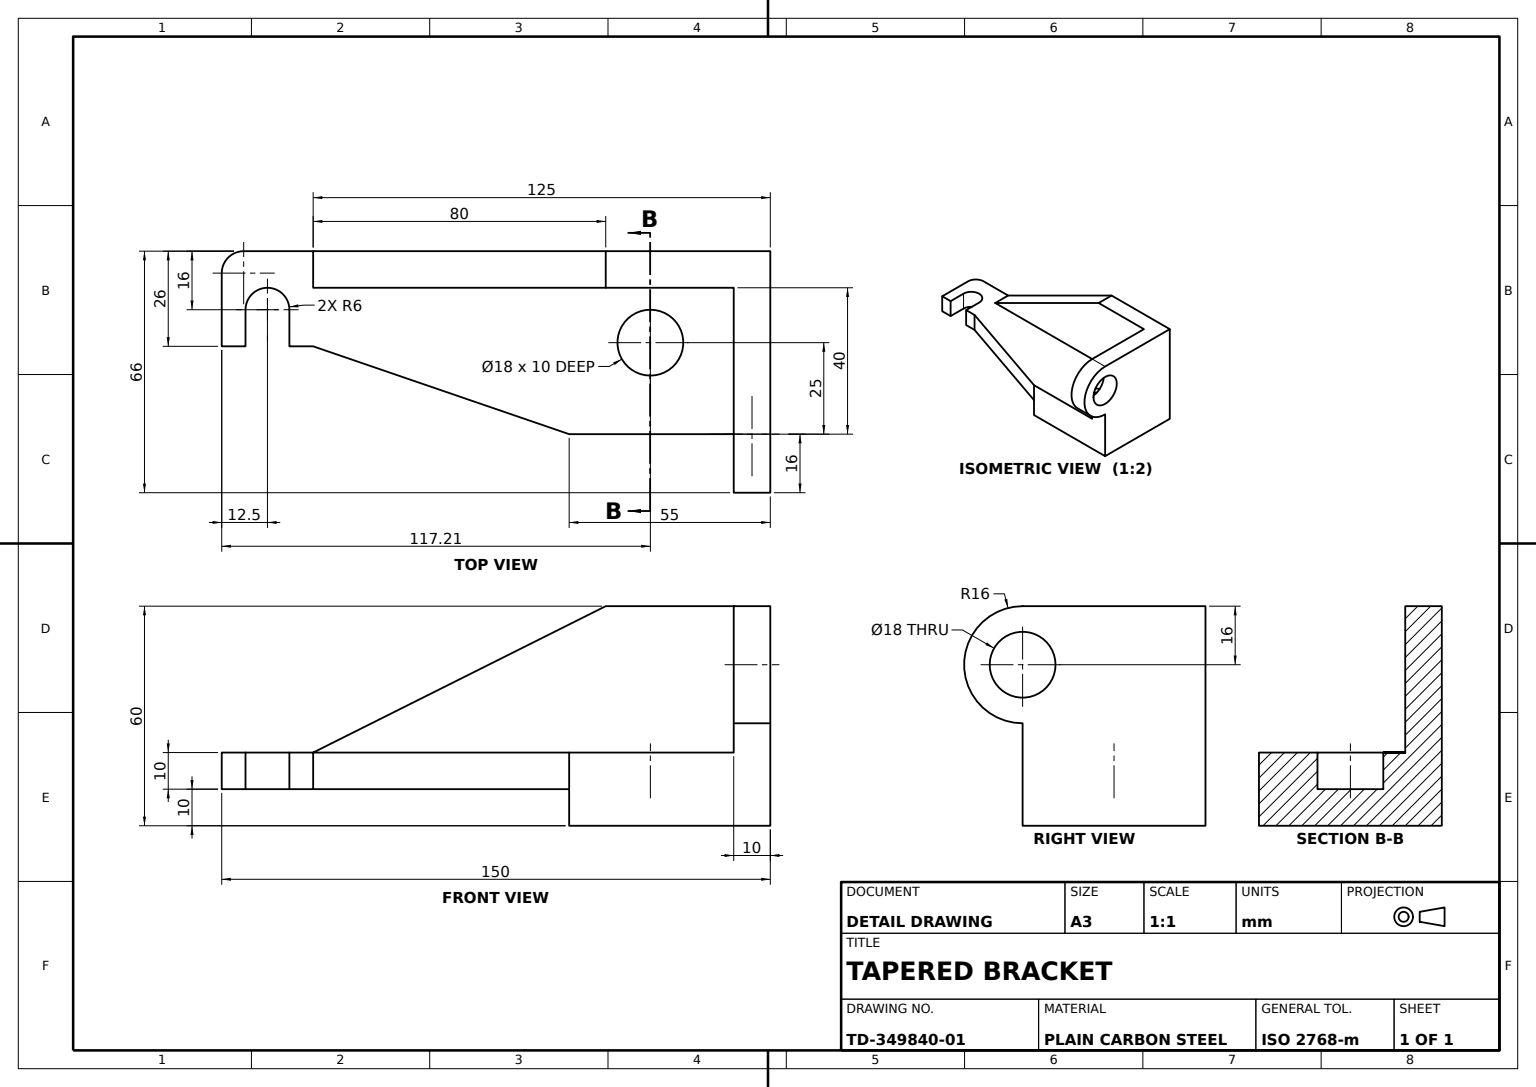
SolidWorks part; units mm, degrees
material "Plain Carbon Steel"
ref_plane "Front Plane" through (0, 0, 0) normal (0, 0, 1) x (1, 0, 0)
ref_plane "Top Plane" through (0, 0, 0) normal (0, 1, 0) x (1, 0, 0)
ref_plane "Right Plane" through (0, 0, 0) normal (1, 0, 0) x (0, 0, -1)
sketch "Base Profile Sketch" plane through (0, 0, 0) normal (0, 0, 1) x (1, 0, 0)
  line L0 (0, 0) -> (125, 0)
  line L1 (125, 0) -> (125, 40)
  line L2 (125, 40) -> (125, 50)
  line L3 (125, 50) -> (80, 50)
  line L4 (80, 50) -> (80, 10)
  line L5 (80, 10) -> (0, 10)
  line L6 (0, 10) -> (0, 0)
  dimension "D1" = 80
  dimension "D2" = 125
  dimension "D3" = 10
  dimension "D4" = 40
extrude "Base Profile" add sketch "Base Profile Sketch" along normal blind 10
sketch "Side Block Sketch" plane through (125, 0, 0) normal (1, 0, 0) x (0, 0, -1)
  line L0 (-10, 50) -> (-60, 50)
  line L1 (-60, 50) -> (-60, 0)
  line L2 (-60, 0) -> (-10, 0)
  line L3 (-10, 0) -> (-10, 50)
extrude "Side Block" add sketch "Side Block Sketch" against normal blind 10
sketch "Web Sketch" plane through (0, 0, 0) normal (0, -1, 0) x (1, 0, 0)
  line L0 (115, 60) -> (70, 60)
  line L1 (0, 10) -> (0, 40)
  line L2 (0, 40) -> (70, 60)
  line L3 (125, 60) -> (125, 0) construction
  line L4 (0, 0) -> (125, 0) construction
  line L9 (0, 0) -> (125, 0)
  line L10 (125, 0) -> (125, 60)
  line L11 (125, 60) -> (115, 60)
  line L12 (115, 60) -> (115, 10)
  line L13 (115, 10) -> (0, 10)
  line L14 (0, 10) -> (0, 0)
  line L18 (115, 60) -> (115, 10)
  line L19 (115, 10) -> (0, 10)
  dimension "D1" = 0
  dimension "D2" = 55
  dimension "D3" = 40
extrude "Web" add sketch "Web Sketch" against normal blind 10
sketch "Gusset Sketch" plane through (0, 0, 0) normal (0, 0, -1) x (-1, 0, 0)
  line L0 (-80, 50) -> (0, 10)
  line L1 (0, 10) -> (-80, 10)
  line L2 (-80, 10) -> (-80, 50)
extrude "Gusset" add sketch "Gusset Sketch" against normal blind 10
sketch "Rail Sketch" plane through (0, 0, 0) normal (0, -1, 0) x (1, 0, 0)
  line L0 (70, 60) -> (125, 60)
  line L1 (125, 60) -> (125, 0)
  line L2 (125, 0) -> (70, 0)
  line L3 (0, 0) -> (125, 0) construction
  line L4 (70, 0) -> (70, 60)
extrude "Rail" add sketch "Rail Sketch" along normal blind 10
sketch "Pocket Cut Sketch" plane through (0, 0, 60) normal (0, 0, 1) x (1, 0, 0)
  line L0 (115, 50) -> (125, 50)
  line L1 (125, 50) -> (125, -10)
  line L2 (125, -10) -> (70, -10)
  line L3 (70, -10) -> (70, 10)
  line L4 (70, 10) -> (115, 10)
  line L5 (115, 10) -> (115, 50)
extrude "Pocket Cut" cut sketch "Pocket Cut Sketch" against normal blind 10
sketch "Relief Cut Sketch" plane through (0, 10, 0) normal (0, 1, 0) x (1, 0, 0)
  line L0 (0, -40) -> (0, -10)
  line L1 (0, -10) -> (70, -10)
  line L2 (0, -10) -> (115, -10) construction
  line L3 (70, -10) -> (70, -60)
  line L4 (70, -60) -> (0, -40)
extrude "Relief Cut" cut sketch "Relief Cut Sketch" against normal blind 10
sketch "Arm Mount Sketch" plane through (0, 10, 0) normal (0, 1, 0) x (1, 0, 0)
  line L0 (70, -10) -> (0, -10)
  line L3 (70, -50) -> (70, -10)
  line L4 (0, -10) -> (0, -26)
  line L5 (0, -26) -> (70, -50)
  line L7 (70, -10) -> (115, -10) construction
  dimension "D1" = 16
extrude "Arm Mount" add sketch "Arm Mount Sketch" against normal blind 10
sketch "Hook Arm Sketch" plane through (0, 0, 0) normal (0, -1, 0) x (1, 0, 0)
  line L0 (0, 0) -> (-19, 0)
  line L1 (-25, 26) -> (-19, 26)
  line L2 (-25, 6) -> (-25, 26)
  line L3 (0, 0) -> (0, 26)
  line L4 (0, 26) -> (-6, 26)
  line L5 (-19, 26) -> (-18.5, 26)
  line L6 (70, 50) -> (70, 0) construction
  line L7 (-18.5, 16) -> (-18.5, 26)
  line L8 (-6.5, 16) -> (-6.5, 26)
  line L9 (-6.5, 26) -> (-6, 26)
  arc A0 (-25, 6) -> (-19, 0) centre (-19, 6) ccw
  arc A1 (-18.5, 16) -> (-6.5, 16) centre (-12.5, 16) ccw
  dimension "D1" = 12
  dimension "D2" = 12
  dimension "D3" = 6
  dimension "D4" = 82.5
  dimension "D5" = 16
extrude "Hook Arm" add sketch "Hook Arm Sketch" against normal blind 10
sketch "Ring Boss Sketch" plane through (125, 0, 0) normal (1, 0, 0) x (0, 0, -1)
  line L0 (-50, 50) -> (-50, 18)
  line L1 (-50, -10) -> (-50, 50) construction
  arc A0 (-50, 50) -> (-50, 18) centre (-50, 34) ccw
  dimension "D1" = 32
  dimension "D2" = 16
extrude "Ring Boss" add sketch "Ring Boss Sketch" against normal blind 10
sketch "Bore Ø18 Sketch" plane through (125, 0, 0) normal (1, 0, 0) x (0, 0, -1)
  circle A0 centre (-50, 34) radius 9
  dimension "D1" = 18
  dimension "D2" = 18
extrude "Bore Ø18" cut sketch "Bore Ø18 Sketch" against normal blind 10
sketch "Hook Cutout Ø18 Sketch" plane through (0, 10, 0) normal (0, 1, 0) x (1, 0, 0)
  line L0 (115, -50) -> (70, -50) construction
  line L1 (-25, -26) -> (-25, -6) construction
  circle A0 centre (92.2059, -25) radius 9
  dimension "D1" = 18
  dimension "D3" = 18
  dimension "D2" = 25
  dimension "D4" = 117.2059
extrude "Hook Cutout Ø18" cut sketch "Hook Cutout Ø18 Sketch" against normal blind 10
